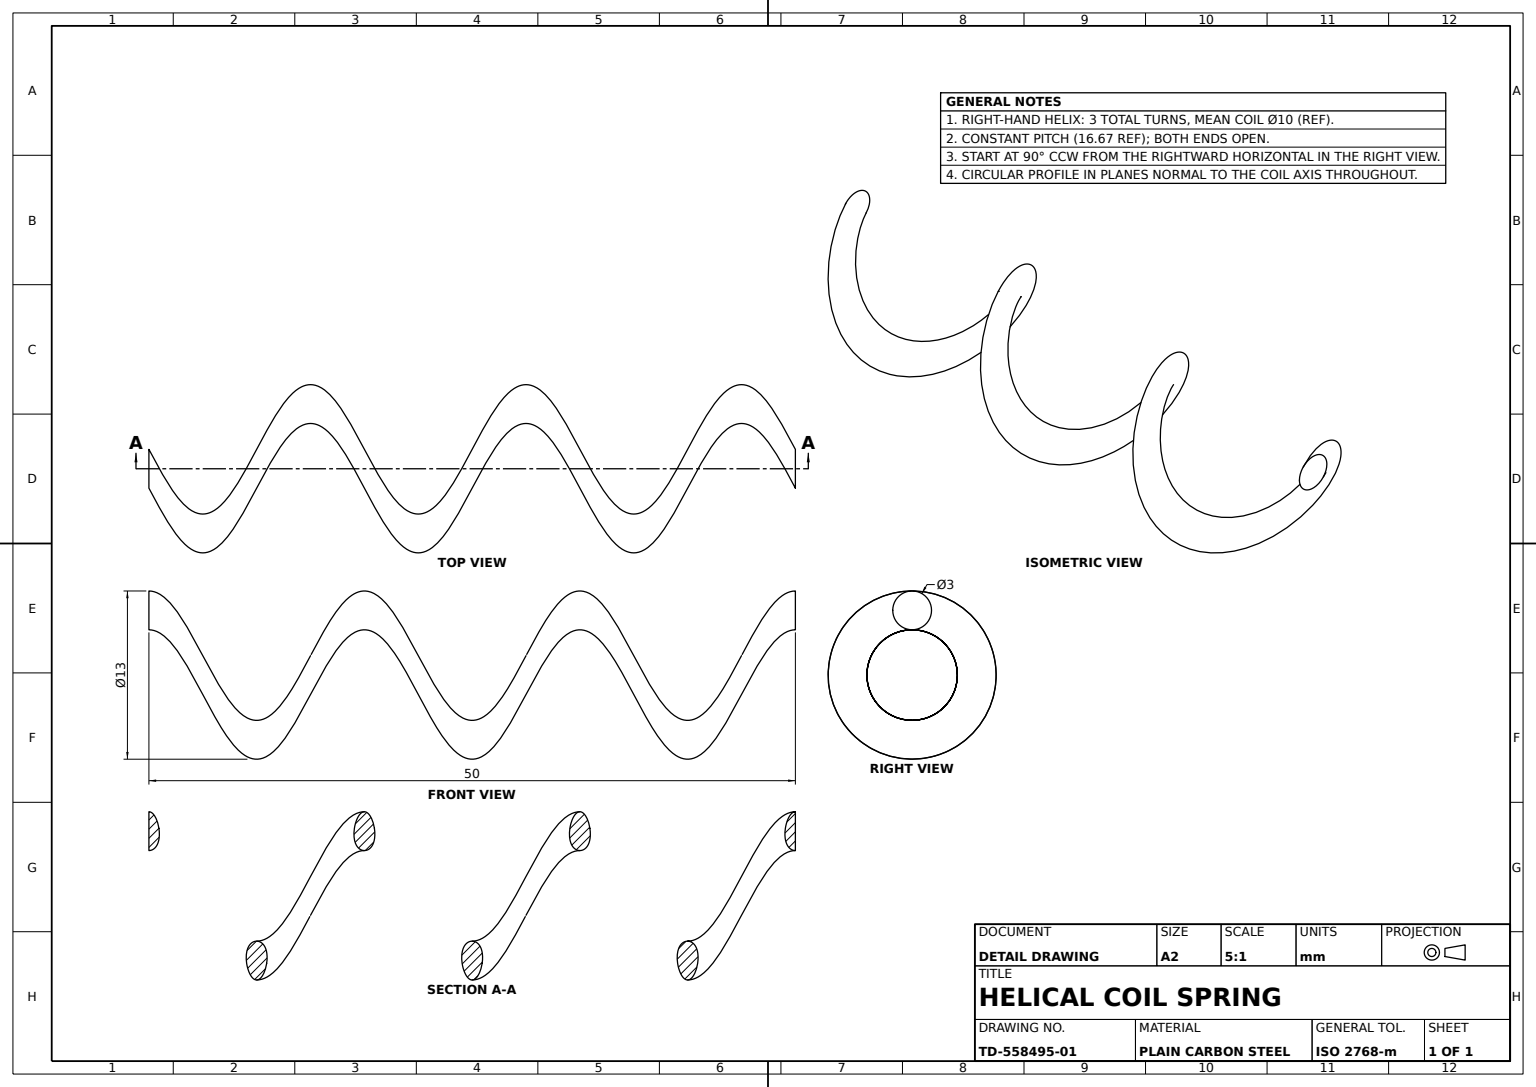
SolidWorks part; units mm, degrees
material "Plain Carbon Steel"
ref_plane "Front Plane" through (0, 0, 0) normal (0, 0, 1) x (1, 0, 0)
ref_plane "Top Plane" through (0, 0, 0) normal (0, 1, 0) x (1, 0, 0)
ref_plane "Right Plane" through (0, 0, 0) normal (1, 0, 0) x (0, 0, -1)
sketch "Coil Base Circle" plane through (0, 0, 0) normal (0, 0, 1) x (1, 0, 0)
  circle A0 centre (0, 0) radius 5
  dimension "D1" = 10
curve "Coil Helix 3 Turns" pitch 16.6667 height 50 turns 3
sketch "Wire Profile" plane through (0, 0, 0) normal (0, 0, 1) x (1, 0, 0)
  circle A0 centre (0, 5) radius 1.5
  dimension "D1" = 3
sweep "Spring Coil" add profiles "Wire Profile" path "Coil Helix 3 Turns"
